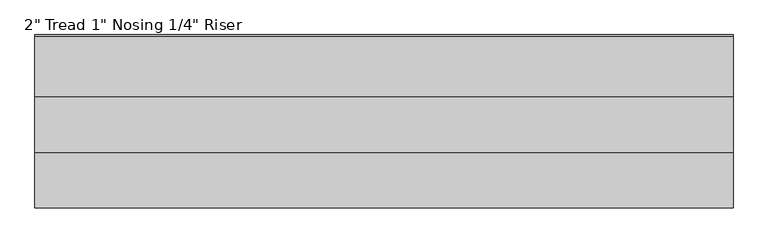
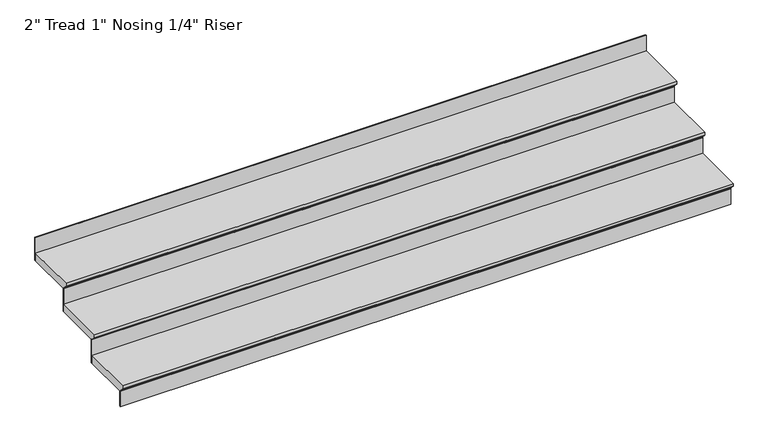
"""IFC4 building model written with IfcOpenShell, lengths in millimetres: stair flight geometry."""

from ifc_helpers import new_model, si_unit, frame, origin, place, context, project, spatial, polyline, outline, extrude, source, transform, mapped, element, save


def stair_flight_523d9302(model_context):
    return source(origin(), model_context, "Body", "SweptSolid", [
        extrude(outline(polyline([(-3700.8806156, -457.2), (-3370.6806156, -457.2), (-3370.6806156, -508.0), (-3675.4806156, -508.0), (-3675.4806156, -501.65), (-3700.8806156, -476.25), (-3700.8806156, -457.2)])), frame((-18891.32252, 0.0, 0.0), z_axis=(1.0, 0.0, 0.0), x_axis=(0.0, 1.0, 0.0)), (0.0, 0.0, 1.0), 3807.2),
        extrude(outline(polyline([(-15084.12252, -3669.1306156), (-15084.12252, -3675.4806156), (-18891.32252, -3675.4806156), (-18891.32252, -3669.1306156), (-15084.12252, -3669.1306156)])), frame((0.0, 0.0, -609.6), z_axis=(0.0, 0.0, 1.0), x_axis=(1.0, 0.0, 0.0)), (0.0, 0.0, 1.0), 101.6),
        extrude(outline(polyline([(-15084.12252, -3364.3306156), (-15084.12252, -3370.6806156), (-18891.32252, -3370.6806156), (-18891.32252, -3364.3306156), (-15084.12252, -3364.3306156)])), frame((0.0, 0.0, -508.0), z_axis=(0.0, 0.0, 1.0), x_axis=(1.0, 0.0, 0.0)), (0.0, 0.0, 1.0), 152.4),
        extrude(outline(polyline([(-3396.0806156, -304.8), (-3065.8806156, -304.8), (-3065.8806156, -355.6), (-3370.6806156, -355.6), (-3370.6806156, -349.25), (-3396.0806156, -323.85), (-3396.0806156, -304.8)])), frame((-18891.32252, 0.0, 0.0), z_axis=(1.0, 0.0, 0.0), x_axis=(0.0, 1.0, 0.0)), (0.0, 0.0, 1.0), 3807.2),
        extrude(outline(polyline([(-15084.12252, -3059.5306156), (-15084.12252, -3065.8806156), (-18891.32252, -3065.8806156), (-18891.32252, -3059.5306156), (-15084.12252, -3059.5306156)])), frame((0.0, 0.0, -355.6), z_axis=(0.0, 0.0, 1.0), x_axis=(1.0, 0.0, 0.0)), (0.0, 0.0, 1.0), 152.4),
        extrude(outline(polyline([(-15084.12252, -2754.7306156), (-15084.12252, -2761.0806156), (-18891.32252, -2761.0806156), (-18891.32252, -2754.7306156), (-15084.12252, -2754.7306156)])), frame((0.0, 0.0, -203.2), z_axis=(0.0, 0.0, 1.0), x_axis=(1.0, 0.0, 0.0)), (0.0, 0.0, 1.0), 152.4),
        extrude(outline(polyline([(-3091.2806156, -152.4), (-2761.0806156, -152.4), (-2761.0806156, -203.2), (-3065.8806156, -203.2), (-3065.8806156, -196.85), (-3091.2806156, -171.45), (-3091.2806156, -152.4)])), frame((-18891.32252, 0.0, 0.0), z_axis=(1.0, 0.0, 0.0), x_axis=(0.0, 1.0, 0.0)), (0.0, 0.0, 1.0), 3807.2),
    ])


if __name__ == "__main__":
    model = new_model("IFC4")
    model_context = context("Model", 3, world=origin())
    ifc_project = project(units=[si_unit("LENGTHUNIT", "METRE", prefix="MILLI")], contexts=[model_context])
    site = spatial("IfcSite", under=ifc_project)
    building = spatial("IfcBuilding", under=site)
    placement = place(None, origin())
    stair_flight_shape = stair_flight_523d9302(model_context)
    element("IfcStairFlight", 1, ObjectType="2\" Tread 1\" Nosing 1/4\" Riser", at=placement, inside=building, context=model_context, shape_type="MappedRepresentation", body=[
        mapped(stair_flight_shape, transform((0.0, 0.0, 0.0), x_axis=(1.0, 0.0, 0.0), y_axis=(0.0, 1.0, 0.0), z_axis=(0.0, 0.0, 1.0))),
    ])
    save(model, "model.ifc")
